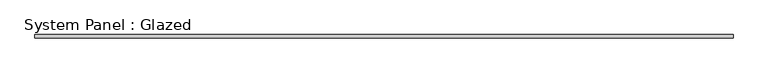
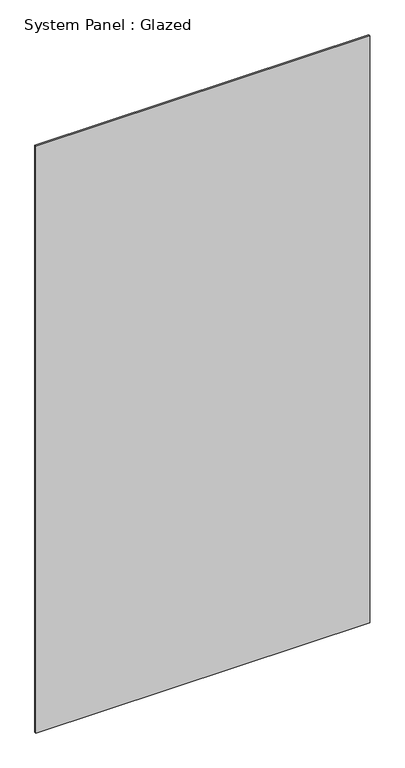
"""IFC4 building model written with IfcOpenShell, lengths in millimetres: plate geometry, System Panel : Glazed."""

from ifc_helpers import new_model, si_unit, origin, origin_with_axes, place, context, project, spatial, polyline, outline, extrude, source, transform, mapped, element, save


def system_panel_glazed_b955046d(model_context):
    return source(origin(), model_context, "Body", "SweptSolid", [
        extrude(outline(polyline([(618.7499999, 34.0), (-618.7499999, 34.0), (-618.7499999, 40.0), (618.7499999, 40.0), (618.7499999, 34.0)])), origin_with_axes(), (0.0, 0.0, 1.0), 2300.0),
    ])


if __name__ == "__main__":
    model = new_model("IFC4")
    model_context = context("Model", 3, world=origin())
    ifc_project = project(units=[si_unit("LENGTHUNIT", "METRE", prefix="MILLI")], contexts=[model_context])
    site = spatial("IfcSite", under=ifc_project)
    building = spatial("IfcBuilding", under=site)
    placement = place(None, origin())
    system_panel_glazed_shape = system_panel_glazed_b955046d(model_context)
    element("IfcPlate", 1, ObjectType="System Panel : Glazed", at=placement, inside=building, context=model_context, shape_type="MappedRepresentation", body=[
        mapped(system_panel_glazed_shape, transform((0.0, 0.0, 0.0), x_axis=(1.0, 0.0, 0.0), y_axis=(0.0, 1.0, 0.0), z_axis=(0.0, 0.0, 1.0))),
    ])
    save(model, "model.ifc")

# Revit data of these elements
# Type "System Panel : Glazed"
#   Construction Type Id = "GSP4R"
#   Analytic Construction = "1/8 in Pilkington single glazing"
#   Visual Light Transmittance = 0.9
#   Solar Heat Gain Coefficient = 0.86
#   Heat Transfer Coefficient (U) = 6.7069 W/(m²·K)
#   Define Thermal Properties by = 1
# Element 1 (IfcPlate, "System Panel : Glazed")
#   Materials on its faces: "Default New Material(6)"
# Materials
#   "Default New Material(6)": class "Generic", colour RGB 191 25 25, transparency 0.9, Cost = 0
